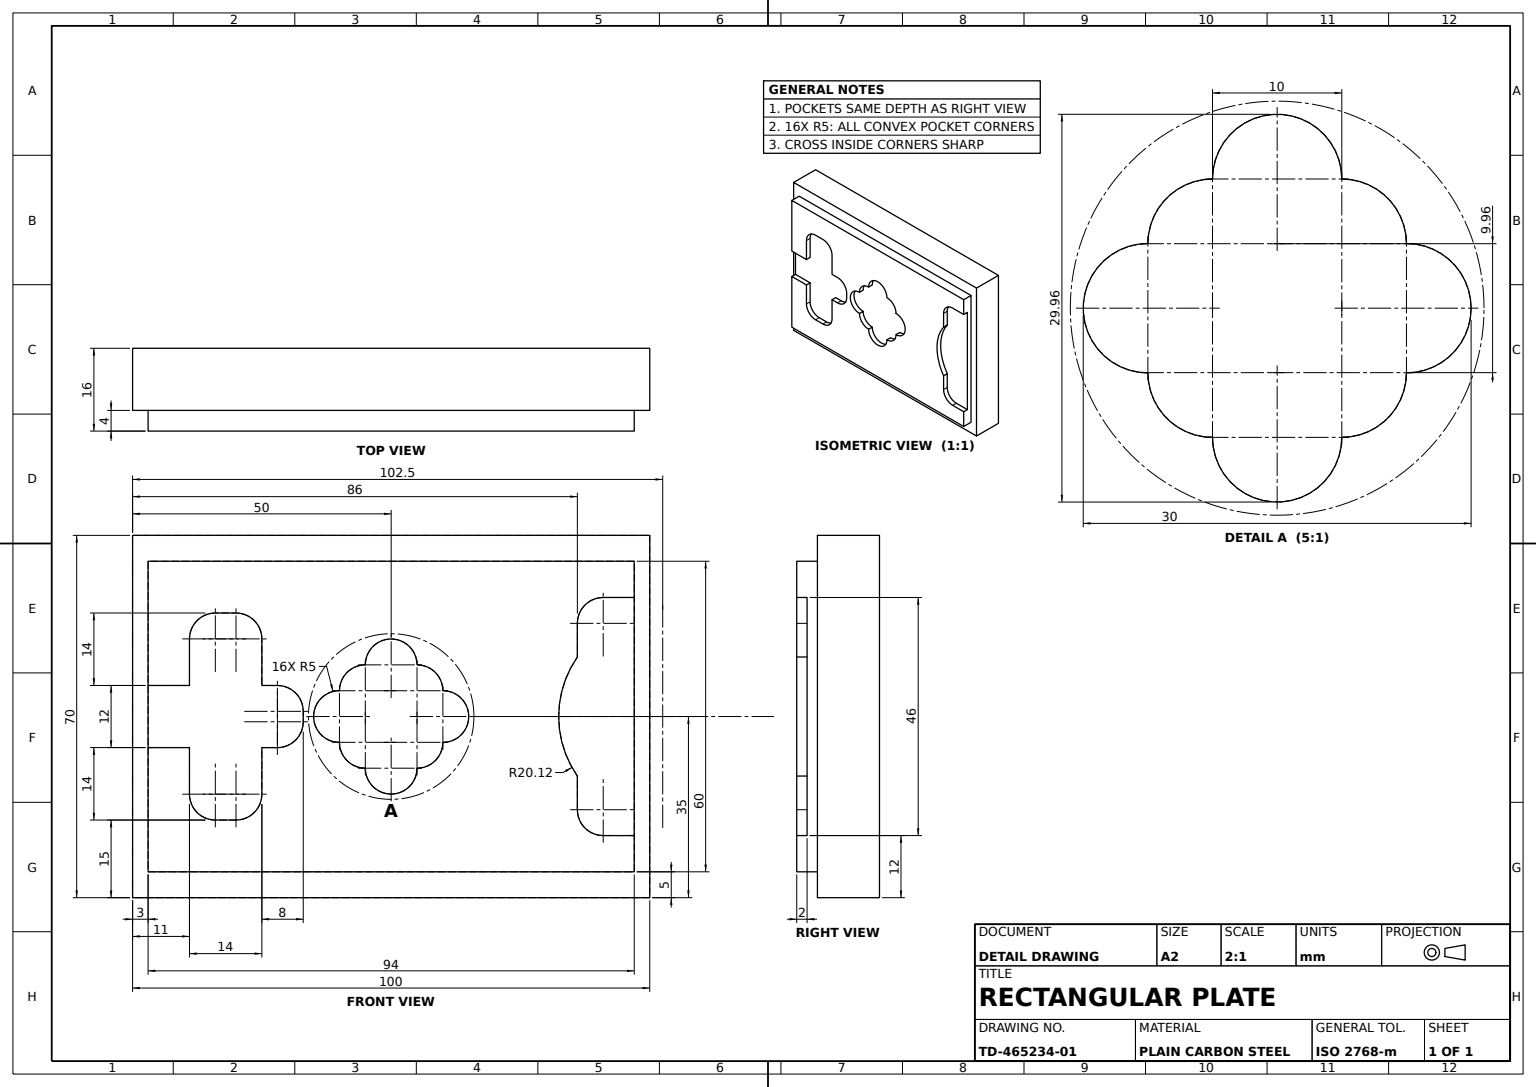
from build123d import *

# Parameters (mm, degrees)
BASE_PLATE_SKETCH_W        = 100
BASE_PLATE_SKETCH_H        = 70
BASE_PLATE_100X70X12_DEPTH = 6
RAISED_PAD_SKETCH_W        = 94
RAISED_PAD_SKETCH_H        = 60
RAISED_PAD_94X60X4_DEPTH   = 4
PAD_CUT_1_DEPTH            = 2
PAD_CUT_2_DEPTH            = 2
PAD_CUT_3_DEPTH            = 2


with BuildPart() as part:
    # Base Plate Sketch → Base Plate 100x70x12 (new, symmetric)
    with BuildSketch(Plane.XY):
        Rectangle(BASE_PLATE_SKETCH_W, BASE_PLATE_SKETCH_H)
    extrude(amount=BASE_PLATE_100X70X12_DEPTH, both=True)

    # Raised Pad Sketch → Raised Pad 94x60x4 (add)
    with BuildSketch(Plane(origin=(0, 0, -6), x_dir=(-1, 0, 0), z_dir=(0, 0, -1))):
        Rectangle(RAISED_PAD_SKETCH_W, RAISED_PAD_SKETCH_H)
    extrude(amount=RAISED_PAD_94X60X4_DEPTH)

    # Pad Cut 1 Sketch → Pad Cut 1 (cut, symmetric)
    with BuildSketch(Plane(origin=(0, 0, -10), x_dir=(-1, 0, 0), z_dir=(0, 0, -1))):
        with BuildLine():
            Line((47, -23), (47, 23))
            Line((47, 23), (41, 23))
            ThreePointArc((41, 23), (37.464466094, 21.535533906), (36, 18))
            Line((36, 18), (36, 11.5))
            ThreePointArc((36, 11.5), (32.388712156, 0), (36, -11.5))
            Line((36, -11.5), (36, -18))
            ThreePointArc((36, -18), (37.464466094, -21.535533906), (41, -23))
            Line((41, -23), (47, -23))
        make_face()
    extrude(amount=PAD_CUT_1_DEPTH, both=True, mode=Mode.SUBTRACT)

    # Pad Cut 2 Sketch → Pad Cut 2 (cut, symmetric)
    with BuildSketch(Plane(origin=(0, 0, -10), x_dir=(-1, 0, 0), z_dir=(0, 0, -1))):
        with BuildLine():
            Line((-47, -6), (-39, -6))
            Line((-39, -6), (-39, -15))
            ThreePointArc((-39, -15), (-37.535533906, -18.535533906), (-34, -20))
            Line((-34, -20), (-30, -20))
            ThreePointArc((-30, -20), (-26.464466094, -18.535533906), (-25, -15))
            Line((-25, -15), (-25, -6))
            Line((-25, -6), (-22.017780858, -6.01060535))
            ThreePointArc((-22.017780858, -6.01060535), (-18.470758176, -4.552451776), (-17, -1.010636966))
            Line((-17, -1.010636966), (-17, 1))
            ThreePointArc((-17, 1), (-18.464466094, 4.535533906), (-22, 6))
            Line((-22, 6), (-25, 6))
            Line((-25, 6), (-25, 15))
            ThreePointArc((-25, 15), (-26.464466094, 18.535533906), (-30, 20))
            Line((-30, 20), (-34, 20))
            ThreePointArc((-34, 20), (-37.535533906, 18.535533906), (-39, 15))
            Line((-39, 15), (-39, 6))
            Line((-39, 6), (-47, 6))
            Line((-47, 6), (-47, -6))
        make_face()
    extrude(amount=PAD_CUT_2_DEPTH, both=True, mode=Mode.SUBTRACT)

    # Pad Cut 3 Sketch → Pad Cut 3 (cut, symmetric)
    with BuildSketch(Plane(origin=(0, 0, -10), x_dir=(-1, 0, 0), z_dir=(0, 0, -1))):
        with BuildLine():
            ThreePointArc((-10, 5.000015487), (-15.000015487, 0), (-10, -5.000015487))
            ThreePointArc((-10, -5.000015487), (-8.529332614, -8.524177957), (-5.000015487, -9.982431809))
            ThreePointArc((-5.000015487, -9.982431809), (0, -14.982447295), (5.000015487, -9.982431809))
            ThreePointArc((5.000015487, -9.982431809), (8.529332614, -8.524177957), (10, -5.000015487))
            ThreePointArc((10, -5.000015487), (15.000015487, 0), (10, 5.000015487))
            ThreePointArc((10, 5.000015487), (8.529332614, 8.524177957), (5.000015487, 9.982431809))
            ThreePointArc((5.000015487, 9.982431809), (0, 14.982447295), (-5.000015487, 9.982431809))
            ThreePointArc((-5.000015487, 9.982431809), (-8.529332614, 8.524177957), (-10, 5.000015487))
        make_face()
    extrude(amount=PAD_CUT_3_DEPTH, both=True, mode=Mode.SUBTRACT)


solid = part.part
